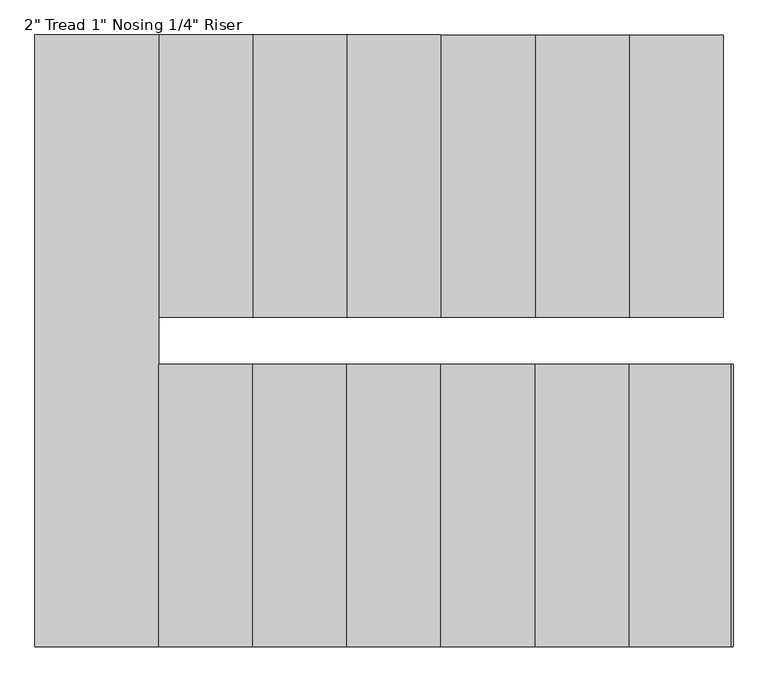
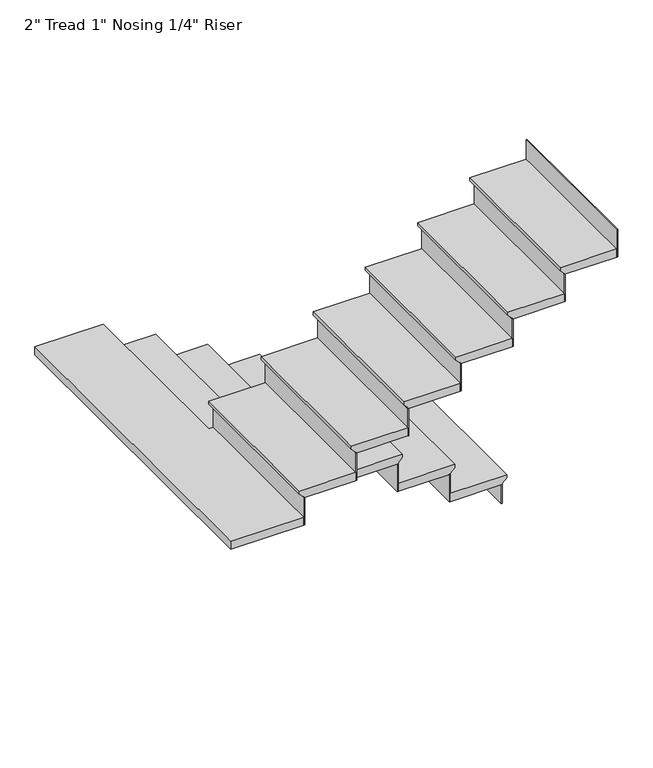
"""IFC4 building model written with IfcOpenShell, lengths in millimetres: stair flight geometry."""

from ifc_helpers import new_model, si_unit, origin, place, context, project, spatial, faceted_brep, source, transform, mapped, element, save


def stair_flight_3e22188b(model_context):
    return source(origin(), model_context, "Body", "Brep", [
        faceted_brep([(3727.9146873, 3708.4, 150.2833333), (3727.9146873, 3708.4, 169.3333333), (3727.9146873, 2794.0, 169.3333333), (3727.9146873, 2794.0, 150.2833333), (3702.5146873, 3708.4, 124.8833333), (3702.5146873, 2794.0, 124.8833333), (3397.7146873, 3708.4, 169.3333333), (3397.7146873, 2794.0, 169.3333333), (3702.5146873, 2794.0, 118.5333333), (3397.7146873, 2794.0, 118.5333333), (3397.7146873, 3708.4, 118.5333333), (3702.5146873, 3708.4, 118.5333333)], [[[0, 1, 2, 3]], [[4, 0, 3, 5]], [[2, 1, 6, 7]], [[8, 9, 10, 11]], [[2, 7, 9, 8, 5, 3]], [[8, 11, 4, 5]], [[6, 1, 0, 4, 11, 10]], [[7, 6, 10, 9]]]),
        faceted_brep([(3702.5146873, 3708.4, 118.5333333), (3702.5146873, 3708.4, 0.0), (3696.1646873, 3708.4, 0.0), (3696.1646873, 3708.4, 118.5333333), (3702.5146873, 2794.0, 118.5333333), (3696.1646873, 2794.0, 118.5333333), (3696.1646873, 2794.0, 0.0), (3702.5146873, 2794.0, 0.0)], [[[0, 1, 2, 3]], [[4, 5, 6, 7]], [[1, 0, 4, 7]], [[2, 1, 7, 6]], [[3, 2, 6, 5]], [[0, 3, 5, 4]]]),
        faceted_brep([(3397.7146873, 3708.4, 287.8666667), (3397.7146873, 3708.4, 118.5333333), (3391.3646873, 3708.4, 118.5333333), (3391.3646873, 3708.4, 287.8666667), (3397.7146873, 2794.0, 287.8666667), (3391.3646873, 2794.0, 287.8666667), (3391.3646873, 2794.0, 118.5333333), (3397.7146873, 2794.0, 118.5333333)], [[[0, 1, 2, 3]], [[4, 5, 6, 7]], [[1, 0, 4, 7]], [[2, 1, 7, 6]], [[3, 2, 6, 5]], [[0, 3, 5, 4]]]),
        faceted_brep([(3423.1146873, 2794.0, 338.6666667), (3423.1146873, 3708.4, 338.6666667), (3092.9146873, 3708.4, 338.6666667), (3092.9146873, 2794.0, 338.6666667), (3397.7146873, 2794.0, 287.8666667), (3092.9146873, 2794.0, 287.8666667), (3092.9146873, 3708.4, 287.8666667), (3397.7146873, 3708.4, 287.8666667), (3397.7146873, 2794.0, 294.2166667), (3423.1146873, 2794.0, 319.6166667), (3397.7146873, 3708.4, 294.2166667), (3423.1146873, 3708.4, 319.6166667)], [[[0, 1, 2, 3]], [[4, 5, 6, 7]], [[0, 3, 5, 4, 8, 9]], [[4, 7, 10, 8]], [[2, 1, 11, 10, 7, 6]], [[3, 2, 6, 5]], [[11, 1, 0, 9]], [[10, 11, 9, 8]]]),
        faceted_brep([(3092.9146873, 3708.4, 457.2), (3092.9146873, 3708.4, 287.8666667), (3086.5646873, 3708.4, 287.8666667), (3086.5646873, 3708.4, 457.2), (3092.9146873, 2794.0, 457.2), (3086.5646873, 2794.0, 457.2), (3086.5646873, 2794.0, 287.8666667), (3092.9146873, 2794.0, 287.8666667)], [[[0, 1, 2, 3]], [[4, 5, 6, 7]], [[1, 0, 4, 7]], [[2, 1, 7, 6]], [[3, 2, 6, 5]], [[0, 3, 5, 4]]]),
        faceted_brep([(3118.3146873, 2794.0, 508.0), (3118.3146873, 3708.4, 508.0), (2788.1146873, 3708.4, 508.0), (2788.1146873, 2794.0, 508.0), (3092.9146873, 2794.0, 457.2), (2788.1146873, 2794.0, 457.2), (2788.1146873, 3708.4, 457.2), (3092.9146873, 3708.4, 457.2), (3092.9146873, 2794.0, 463.55), (3118.3146873, 2794.0, 488.95), (3092.9146873, 3708.4, 463.55), (3118.3146873, 3708.4, 488.95)], [[[0, 1, 2, 3]], [[4, 5, 6, 7]], [[0, 3, 5, 4, 8, 9]], [[4, 7, 10, 8]], [[2, 1, 11, 10, 7, 6]], [[3, 2, 6, 5]], [[11, 1, 0, 9]], [[10, 11, 9, 8]]]),
        faceted_brep([(2788.1146873, 3708.4, 626.5333333), (2788.1146873, 3708.4, 457.2), (2781.7646873, 3708.4, 457.2), (2781.7646873, 3708.4, 626.5333333), (2788.1146873, 2794.0, 626.5333333), (2781.7646873, 2794.0, 626.5333333), (2781.7646873, 2794.0, 457.2), (2788.1146873, 2794.0, 457.2)], [[[0, 1, 2, 3]], [[4, 5, 6, 7]], [[1, 0, 4, 7]], [[2, 1, 7, 6]], [[3, 2, 6, 5]], [[0, 3, 5, 4]]]),
        faceted_brep([(2813.5146873, 2794.0, 677.3333333), (2813.5146873, 3708.4, 677.3333333), (2483.3146873, 3708.4, 677.3333333), (2483.3146873, 2794.0, 677.3333333), (2788.1146873, 2794.0, 626.5333333), (2483.3146873, 2794.0, 626.5333333), (2483.3146873, 3708.4, 626.5333333), (2788.1146873, 3708.4, 626.5333333), (2788.1146873, 2794.0, 632.8833333), (2813.5146873, 2794.0, 658.2833333), (2788.1146873, 3708.4, 632.8833333), (2813.5146873, 3708.4, 658.2833333)], [[[0, 1, 2, 3]], [[4, 5, 6, 7]], [[0, 3, 5, 4, 8, 9]], [[4, 7, 10, 8]], [[2, 1, 11, 10, 7, 6]], [[3, 2, 6, 5]], [[11, 1, 0, 9]], [[10, 11, 9, 8]]]),
        faceted_brep([(2483.3146873, 3708.4, 795.8666667), (2483.3146873, 3708.4, 626.5333333), (2476.9646873, 3708.4, 626.5333333), (2476.9646873, 3708.4, 795.8666667), (2483.3146873, 2794.0, 795.8666667), (2476.9646873, 2794.0, 795.8666667), (2476.9646873, 2794.0, 626.5333333), (2483.3146873, 2794.0, 626.5333333)], [[[0, 1, 2, 3]], [[4, 5, 6, 7]], [[1, 0, 4, 7]], [[2, 1, 7, 6]], [[3, 2, 6, 5]], [[0, 3, 5, 4]]]),
        faceted_brep([(2508.7146873, 2794.0, 846.6666667), (2508.7146873, 3708.4, 846.6666667), (2178.5146873, 3708.4, 846.6666667), (2178.5146873, 2794.0, 846.6666667), (2483.3146873, 2794.0, 795.8666667), (2178.5146873, 2794.0, 795.8666667), (2178.5146873, 3708.4, 795.8666667), (2483.3146873, 3708.4, 795.8666667), (2483.3146873, 2794.0, 802.2166667), (2508.7146873, 2794.0, 827.6166667), (2483.3146873, 3708.4, 802.2166667), (2508.7146873, 3708.4, 827.6166667)], [[[0, 1, 2, 3]], [[4, 5, 6, 7]], [[0, 3, 5, 4, 8, 9]], [[4, 7, 10, 8]], [[2, 1, 11, 10, 7, 6]], [[3, 2, 6, 5]], [[11, 1, 0, 9]], [[10, 11, 9, 8]]]),
        faceted_brep([(2178.5146873, 3708.4, 965.2), (2178.5146873, 3708.4, 795.8666667), (2172.1646873, 3708.4, 795.8666667), (2172.1646873, 3708.4, 965.2), (2178.5146873, 2794.0, 965.2), (2172.1646873, 2794.0, 965.2), (2172.1646873, 2794.0, 795.8666667), (2178.5146873, 2794.0, 795.8666667)], [[[0, 1, 2, 3]], [[4, 5, 6, 7]], [[1, 0, 4, 7]], [[2, 1, 7, 6]], [[3, 2, 6, 5]], [[0, 3, 5, 4]]]),
        faceted_brep([(2203.9146873, 2794.0, 1016.0), (2203.9146873, 3708.4, 1016.0), (1873.7146873, 3708.4, 1016.0), (1873.7146873, 2794.0, 1016.0), (2178.5146873, 2794.0, 965.2), (1873.7146873, 2794.0, 965.2), (1873.7146873, 3708.4, 965.2), (2178.5146873, 3708.4, 965.2), (2178.5146873, 2794.0, 971.55), (2203.9146873, 2794.0, 996.95), (2178.5146873, 3708.4, 971.55), (2203.9146873, 3708.4, 996.95)], [[[0, 1, 2, 3]], [[4, 5, 6, 7]], [[0, 3, 5, 4, 8, 9]], [[4, 7, 10, 8]], [[2, 1, 11, 10, 7, 6]], [[3, 2, 6, 5]], [[11, 1, 0, 9]], [[10, 11, 9, 8]]]),
        faceted_brep([(1873.7146873, 3708.4, 1134.5333333), (1873.7146873, 3708.4, 965.2), (1867.3646873, 3708.4, 965.2), (1867.3646873, 3708.4, 1134.5333333), (1873.7146873, 2794.0, 1134.5333333), (1867.3646873, 2794.0, 1134.5333333), (1867.3646873, 2794.0, 965.2), (1873.7146873, 2794.0, 965.2)], [[[0, 1, 2, 3]], [[4, 5, 6, 7]], [[1, 0, 4, 7]], [[2, 1, 7, 6]], [[3, 2, 6, 5]], [[0, 3, 5, 4]]]),
        faceted_brep([(1924.5146873, 2641.6, 1185.3333333), (1899.1146873, 2641.6, 1185.3333333), (1899.1146873, 3708.4, 1185.3333333), (1498.6, 3708.4, 1185.3333333), (1498.6, 1727.2, 1185.3333333), (1924.5146873, 1727.2, 1185.3333333), (1899.1146873, 2641.6, 1134.5333333), (1924.5146873, 2641.6, 1134.5333333), (1924.5146873, 1727.2, 1134.5333333), (1498.6, 1727.2, 1134.5333333), (1498.6, 3708.4, 1134.5333333), (1873.7146873, 3708.4, 1134.5333333), (1873.7146873, 2794.0, 1134.5333333), (1899.1146873, 2794.0, 1134.5333333), (1899.1146873, 2794.0, 1166.2833333), (1899.1146873, 3708.4, 1166.2833333), (1873.7146873, 2794.0, 1140.8833333), (1873.7146873, 3708.4, 1140.8833333)], [[[0, 1, 2, 3, 4, 5]], [[6, 7, 8, 9, 10, 11, 12, 13]], [[1, 0, 7, 6]], [[2, 1, 6, 13, 14, 15]], [[13, 12, 16, 14]], [[12, 11, 17, 16]], [[3, 2, 15, 17, 11, 10]], [[4, 3, 10, 9]], [[5, 4, 9, 8]], [[0, 5, 8, 7]], [[17, 15, 14, 16]]]),
        faceted_brep([(1924.5146873, 1727.2, 1303.8666667), (1924.5146873, 1727.2, 1134.5333333), (1930.8646873, 1727.2, 1134.5333333), (1930.8646873, 1727.2, 1303.8666667), (1924.5146873, 2641.6, 1303.8666667), (1930.8646873, 2641.6, 1303.8666667), (1930.8646873, 2641.6, 1134.5333333), (1924.5146873, 2641.6, 1134.5333333)], [[[0, 1, 2, 3]], [[4, 5, 6, 7]], [[1, 0, 4, 7]], [[2, 1, 7, 6]], [[3, 2, 6, 5]], [[0, 3, 5, 4]]]),
        faceted_brep([(1899.1146873, 2641.6, 1354.6666667), (1899.1146873, 1727.2, 1354.6666667), (2229.3146873, 1727.2, 1354.6666667), (2229.3146873, 2641.6, 1354.6666667), (1924.5146873, 2641.6, 1303.8666667), (2229.3146873, 2641.6, 1303.8666667), (2229.3146873, 1727.2, 1303.8666667), (1924.5146873, 1727.2, 1303.8666667), (1924.5146873, 2641.6, 1310.2166667), (1899.1146873, 2641.6, 1335.6166667), (1924.5146873, 1727.2, 1310.2166667), (1899.1146873, 1727.2, 1335.6166667)], [[[0, 1, 2, 3]], [[4, 5, 6, 7]], [[0, 3, 5, 4, 8, 9]], [[4, 7, 10, 8]], [[2, 1, 11, 10, 7, 6]], [[3, 2, 6, 5]], [[11, 1, 0, 9]], [[10, 11, 9, 8]]]),
        faceted_brep([(2229.3146873, 1727.2, 1473.2), (2229.3146873, 1727.2, 1303.8666667), (2235.6646873, 1727.2, 1303.8666667), (2235.6646873, 1727.2, 1473.2), (2229.3146873, 2641.6, 1473.2), (2235.6646873, 2641.6, 1473.2), (2235.6646873, 2641.6, 1303.8666667), (2229.3146873, 2641.6, 1303.8666667)], [[[0, 1, 2, 3]], [[4, 5, 6, 7]], [[1, 0, 4, 7]], [[2, 1, 7, 6]], [[3, 2, 6, 5]], [[0, 3, 5, 4]]]),
        faceted_brep([(2203.9146873, 2641.6, 1524.0), (2203.9146873, 1727.2, 1524.0), (2534.1146873, 1727.2, 1524.0), (2534.1146873, 2641.6, 1524.0), (2229.3146873, 2641.6, 1473.2), (2534.1146873, 2641.6, 1473.2), (2534.1146873, 1727.2, 1473.2), (2229.3146873, 1727.2, 1473.2), (2229.3146873, 2641.6, 1479.55), (2203.9146873, 2641.6, 1504.95), (2229.3146873, 1727.2, 1479.55), (2203.9146873, 1727.2, 1504.95)], [[[0, 1, 2, 3]], [[4, 5, 6, 7]], [[0, 3, 5, 4, 8, 9]], [[4, 7, 10, 8]], [[2, 1, 11, 10, 7, 6]], [[3, 2, 6, 5]], [[11, 1, 0, 9]], [[10, 11, 9, 8]]]),
        faceted_brep([(2534.1146873, 1727.2, 1642.5333333), (2534.1146873, 1727.2, 1473.2), (2540.4646873, 1727.2, 1473.2), (2540.4646873, 1727.2, 1642.5333333), (2534.1146873, 2641.6, 1642.5333333), (2540.4646873, 2641.6, 1642.5333333), (2540.4646873, 2641.6, 1473.2), (2534.1146873, 2641.6, 1473.2)], [[[0, 1, 2, 3]], [[4, 5, 6, 7]], [[1, 0, 4, 7]], [[2, 1, 7, 6]], [[3, 2, 6, 5]], [[0, 3, 5, 4]]]),
        faceted_brep([(2508.7146873, 2641.6, 1693.3333333), (2508.7146873, 1727.2, 1693.3333333), (2838.9146873, 1727.2, 1693.3333333), (2838.9146873, 2641.6, 1693.3333333), (2534.1146873, 2641.6, 1642.5333333), (2838.9146873, 2641.6, 1642.5333333), (2838.9146873, 1727.2, 1642.5333333), (2534.1146873, 1727.2, 1642.5333333), (2534.1146873, 2641.6, 1648.8833333), (2508.7146873, 2641.6, 1674.2833333), (2534.1146873, 1727.2, 1648.8833333), (2508.7146873, 1727.2, 1674.2833333)], [[[0, 1, 2, 3]], [[4, 5, 6, 7]], [[0, 3, 5, 4, 8, 9]], [[4, 7, 10, 8]], [[2, 1, 11, 10, 7, 6]], [[3, 2, 6, 5]], [[11, 1, 0, 9]], [[10, 11, 9, 8]]]),
        faceted_brep([(2838.9146873, 1727.2, 1811.8666667), (2838.9146873, 1727.2, 1642.5333333), (2845.2646873, 1727.2, 1642.5333333), (2845.2646873, 1727.2, 1811.8666667), (2838.9146873, 2641.6, 1811.8666667), (2845.2646873, 2641.6, 1811.8666667), (2845.2646873, 2641.6, 1642.5333333), (2838.9146873, 2641.6, 1642.5333333)], [[[0, 1, 2, 3]], [[4, 5, 6, 7]], [[1, 0, 4, 7]], [[2, 1, 7, 6]], [[3, 2, 6, 5]], [[0, 3, 5, 4]]]),
        faceted_brep([(2813.5146873, 2641.6, 1862.6666667), (2813.5146873, 1727.2, 1862.6666667), (3143.7146873, 1727.2, 1862.6666667), (3143.7146873, 2641.6, 1862.6666667), (2838.9146873, 2641.6, 1811.8666667), (3143.7146873, 2641.6, 1811.8666667), (3143.7146873, 1727.2, 1811.8666667), (2838.9146873, 1727.2, 1811.8666667), (2838.9146873, 2641.6, 1818.2166667), (2813.5146873, 2641.6, 1843.6166667), (2838.9146873, 1727.2, 1818.2166667), (2813.5146873, 1727.2, 1843.6166667)], [[[0, 1, 2, 3]], [[4, 5, 6, 7]], [[0, 3, 5, 4, 8, 9]], [[4, 7, 10, 8]], [[2, 1, 11, 10, 7, 6]], [[3, 2, 6, 5]], [[11, 1, 0, 9]], [[10, 11, 9, 8]]]),
        faceted_brep([(3143.7146873, 1727.2, 1981.2), (3143.7146873, 1727.2, 1811.8666667), (3150.0646873, 1727.2, 1811.8666667), (3150.0646873, 1727.2, 1981.2), (3143.7146873, 2641.6, 1981.2), (3150.0646873, 2641.6, 1981.2), (3150.0646873, 2641.6, 1811.8666667), (3143.7146873, 2641.6, 1811.8666667)], [[[0, 1, 2, 3]], [[4, 5, 6, 7]], [[1, 0, 4, 7]], [[2, 1, 7, 6]], [[3, 2, 6, 5]], [[0, 3, 5, 4]]]),
        faceted_brep([(3118.3146873, 2641.6, 2032.0), (3118.3146873, 1727.2, 2032.0), (3448.5146873, 1727.2, 2032.0), (3448.5146873, 2641.6, 2032.0), (3143.7146873, 2641.6, 1981.2), (3448.5146873, 2641.6, 1981.2), (3448.5146873, 1727.2, 1981.2), (3143.7146873, 1727.2, 1981.2), (3143.7146873, 2641.6, 1987.55), (3118.3146873, 2641.6, 2012.95), (3143.7146873, 1727.2, 1987.55), (3118.3146873, 1727.2, 2012.95)], [[[0, 1, 2, 3]], [[4, 5, 6, 7]], [[0, 3, 5, 4, 8, 9]], [[4, 7, 10, 8]], [[2, 1, 11, 10, 7, 6]], [[3, 2, 6, 5]], [[11, 1, 0, 9]], [[10, 11, 9, 8]]]),
        faceted_brep([(3448.5146873, 1727.2, 2150.5333333), (3448.5146873, 1727.2, 1981.2), (3454.8646873, 1727.2, 1981.2), (3454.8646873, 1727.2, 2150.5333333), (3448.5146873, 2641.6, 2150.5333333), (3454.8646873, 2641.6, 2150.5333333), (3454.8646873, 2641.6, 1981.2), (3448.5146873, 2641.6, 1981.2)], [[[0, 1, 2, 3]], [[4, 5, 6, 7]], [[1, 0, 4, 7]], [[2, 1, 7, 6]], [[3, 2, 6, 5]], [[0, 3, 5, 4]]]),
        faceted_brep([(3753.3146873, 1727.2, 2319.8666667), (3753.3146873, 1727.2, 2150.5333333), (3759.6646873, 1727.2, 2150.5333333), (3759.6646873, 1727.2, 2319.8666667), (3753.3146873, 2641.6, 2319.8666667), (3759.6646873, 2641.6, 2319.8666667), (3759.6646873, 2641.6, 2150.5333333), (3753.3146873, 2641.6, 2150.5333333)], [[[0, 1, 2, 3]], [[4, 5, 6, 7]], [[1, 0, 4, 7]], [[2, 1, 7, 6]], [[3, 2, 6, 5]], [[0, 3, 5, 4]]]),
        faceted_brep([(3423.1146873, 2641.6, 2201.3333333), (3423.1146873, 1727.2, 2201.3333333), (3753.3146873, 1727.2, 2201.3333333), (3753.3146873, 2641.6, 2201.3333333), (3448.5146873, 2641.6, 2150.5333333), (3753.3146873, 2641.6, 2150.5333333), (3753.3146873, 1727.2, 2150.5333333), (3448.5146873, 1727.2, 2150.5333333), (3448.5146873, 2641.6, 2156.8833333), (3423.1146873, 2641.6, 2182.2833333), (3448.5146873, 1727.2, 2156.8833333), (3423.1146873, 1727.2, 2182.2833333)], [[[0, 1, 2, 3]], [[4, 5, 6, 7]], [[0, 3, 5, 4, 8, 9]], [[4, 7, 10, 8]], [[2, 1, 11, 10, 7, 6]], [[3, 2, 6, 5]], [[11, 1, 0, 9]], [[10, 11, 9, 8]]]),
    ])


if __name__ == "__main__":
    model = new_model("IFC4")
    model_context = context("Model", 3, world=origin())
    ifc_project = project(units=[si_unit("LENGTHUNIT", "METRE", prefix="MILLI")], contexts=[model_context])
    site = spatial("IfcSite", under=ifc_project)
    building = spatial("IfcBuilding", under=site)
    placement = place(None, origin())
    stair_flight_shape = stair_flight_3e22188b(model_context)
    element("IfcStairFlight", 1, ObjectType="2\" Tread 1\" Nosing 1/4\" Riser", at=placement, inside=building, context=model_context, shape_type="MappedRepresentation", body=[
        mapped(stair_flight_shape, transform((0.0, 0.0, 0.0), x_axis=(1.0, 0.0, 0.0), y_axis=(0.0, 1.0, 0.0), z_axis=(0.0, 0.0, 1.0))),
    ])
    save(model, "model.ifc")
